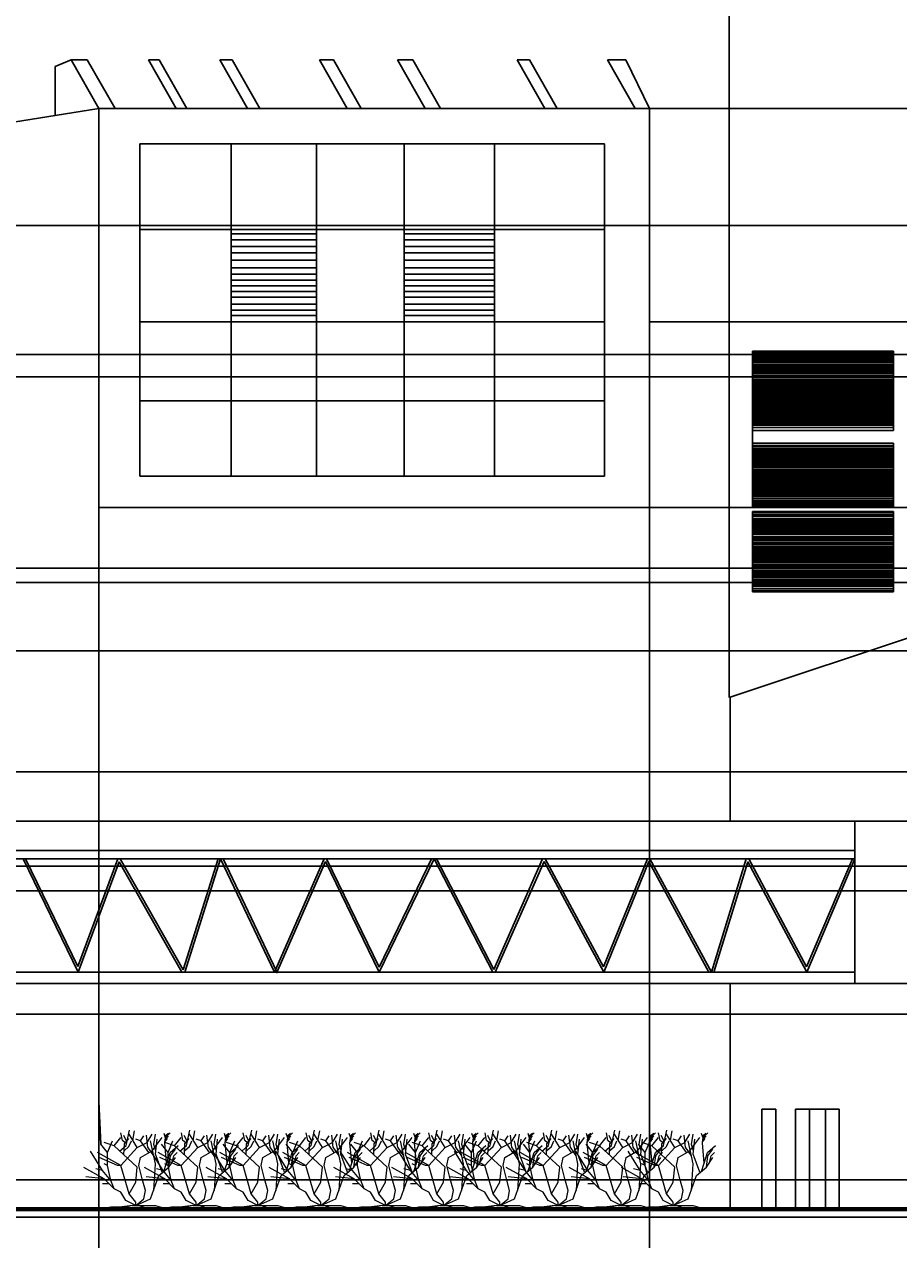
# Model space of a CAD drawing. Units: inches. Extents: x -32109 to 33221, y -19197 to 7608.
# Tile 20 of 25: x 12337 to 15375, y -2226 to 1998. Entities that reach past the tile are written whole.
import ezdxf

# ---------------------------------------------------------------- set-up
doc = ezdxf.new("R2010")
doc.units = ezdxf.units.IN
doc.header["$MEASUREMENT"] = 0
for name, color, linetype, lineweight in [('A-ANNO-DIMS', 2, 'Continuous', 18), ('A-ELEV', 7, 'Continuous', 25), ('L-PLNT', 3, 'Continuous', 13)]:
    doc.layers.add(name, color=color, linetype=linetype, lineweight=lineweight)
doc.styles.get("Standard").update_dxf_attribs({"font": 'arial.ttf'})
doc.dimstyles.get("Standard").update_dxf_attribs({"dimtxt": 0.18, "dimasz": 0.18, "dimexe": 0.18, "dimexo": 0.0625, "dimgap": 0.09, "dimtad": 0, "dimtih": 1, "dimtoh": 1, "dimdec": 4, "dimzin": 0, "dimdsep": 46, "dimtxsty": 'Standard', "dimcen": 0.09, "dimadec": 0, "dimazin": 0, "dimtfac": 1, "dimtdec": 4, "dimtofl": 0, "dimtmove": 0, "dimatfit": 3, "dimfxl": 1, "dimtolj": 1, "dimtzin": 0, "dimarcsym": 0})

# ---------------------------------------------------------------- blocks, each defined once
blk = doc.blocks.new('*U3')
for p, q in [((-12.471, 19.775), (-12.898, 22.044)), ((-11.28, 19.619), (-12.104, 21.184)), ((-11.433, 18.289), (-10.457, 22.749)), ((-8.16, 17.76), (-10.56, 21.6)), ((-9.48, 19.775), (-8.992, 22.592)), ((-5.086, 17.741), (-5.513, 21.34)), ((-5.28, 19.2), (-3.84, 21.6)), ((-3.377, 18.602), (-2.888, 21.575)), ((-0.508, 21.888), (-0.081, 20.558)), ((-0.203, 19.149), (0.102, 21.34)), ((0.041, 20.714), (1.384, 22.044)), ((0.102, 21.34), (0.835, 21.888)), ((-16.8, 16.32), (-18.72, 18.72)), ((-14.88, 18.24), (-17.76, 19.2)), ((-16.8, 16.32), (-15.36, 19.68)), ((-14.88, 18.24), (-12.96, 20.64)), ((-8.16, 12), (-14.88, 18.24)), ((-13.325, 16.724), (-11.433, 18.289)), ((-12.96, 12.48), (-8.16, 17.76)), ((-11.677, 19.071), (-12.471, 19.775)), ((-12.043, 15.628), (-11.921, 18.836)), ((-11.982, 16.802), (-10.579, 18.054)), ((-11.921, 18.836), (-10.64, 20.401)), ((-10.579, 18.054), (-9.846, 19.697)), ((-7.2, 19.68), (-8.64, 20.16)), ((-8.16, 17.76), (-5.28, 19.2)), ((-7.2, 19.68), (-6.24, 21.12)), ((-4.8, 16.32), (-7.2, 19.68)), ((-3.377, 15.315), (-5.086, 17.819)), ((-2.88, 12.96), (-4.32, 19.68)), ((-3.84, 16.8), (-0.96, 20.64)), ((-2.766, 16.802), (-3.377, 18.602)), ((-2.88, 15.84), (-2.4, 20.16)), ((0.346, 13.203), (-0.203, 19.149)), ((-0.142, 19.384), (0.59, 20.401)), ((-0.02, 20.01), (0.896, 21.105)), ((1.323, 16.254), (3.642, 18.289)), ((-18.24, 11.04), (-21.755, 16.655)), ((-12.96, 12.48), (-19.68, 16.32)), ((-13.92, 12.48), (-19.2, 14.88)), ((-16.8, 12.48), (-16.8, 16.32)), ((-7.68, 12.48), (-7.2, 14.88)), ((-7.2, 14.88), (-3.84, 16.8)), ((-0.96, 10.56), (-2.88, 15.84)), ((0.346, 13.203), (1.323, 16.254)), ((0.96, 12), (1.44, 15.36)), ((0.96, 12), (2.88, 14.88)), ((1.44, 15.36), (2.88, 17.28)), ((1.92, 13.44), (2.4, 15.36)), ((2.4, 15.36), (3.36, 16.32)), ((-17.76, 8.64), (-23.663, 11.961)), ((-18.24, 11.04), (-20.16, 11.52)), ((-15.84, 8.16), (-18.24, 11.04)), ((-16.8, 12.48), (-17.76, 12.96)), ((-15.84, 8.16), (-16.8, 12.48)), ((-12.96, 12.48), (-13.92, 12.48)), ((-10.56, 4.32), (-12.96, 12.48)), ((-8.64, 7.68), (-8.16, 12)), ((-6.72, 8.64), (-7.68, 12.48)), ((-3.36, 5.28), (-2.88, 12.96)), ((-1.92, 9.6), (0.96, 12)), ((-0.48, 10.8), (0.346, 13.203)), ((-17.76, 8.64), (-23.128, 9.222)), ((-16.32, 7.2), (-18.24, 7.2)), ((-14.88, 5.76), (-17.76, 8.64)), ((-14.88, 5.76), (-15.84, 8.16)), ((-10.56, 4.32), (-8.64, 7.68)), ((-5.76, 5.28), (-6.72, 8.64)), ((-4.32, 2.88), (-1.92, 9.6)), ((-12.96, 4.8), (-14.88, 5.76)), ((-11.52, 2.4), (-12.96, 4.8)), ((-8.64, 1.92), (-10.56, 4.32)), ((-6.24, 2.88), (-5.76, 5.28)), ((-15.84, 0.48), (-17.76, 0)), ((-13.44, 0.48), (-15.84, 0.48)), ((-9.6, 0.96), (-13.44, 0.48)), ((-9.6, 0.96), (-12.96, 0)), ((-8.64, 0.96), (-11.52, 2.4)), ((-9.6, 0.96), (-7.68, 0.96)), ((-8.64, 0.96), (-4.32, 2.88)), ((-8.64, 0.96), (-6.24, 2.88)), ((-8.64, 0.96), (-8.64, 1.92)), ((-8.64, 0.96), (-2.88, 0.96)), ((-7.68, 0.96), (-6.24, 0.48)), ((-6.24, 0.48), (-3.36, 0)), ((-2.88, 0.96), (0, 0))]:
    blk.add_line(p, q)
blk = doc.blocks.new('*D10')
at = {"layer": 'A-ANNO-DIMS', "color": 0, "lineweight": -2, "transparency": 16777216}
for p, q in [((-18512.6, -110.2), (-18512.6, 5772)), ((-18512.5, 5771.8), (-202.1, 5771.8)), ((18109.1, 5771.8), (-201.2, 5771.8)), ((18109.3, -101.5), (18109.3, 5772))]:
    blk.add_line(p, q, dxfattribs=at)
at = {"layer": 'A-ANNO-DIMS', "color": 0, "transparency": 16777216}
for points in [[(-18512.5, 5771.9), (-18512.5, 5771.8), (-18512.6, 5771.8)], [(18109.1, 5771.9), (18109.1, 5771.8), (18109.3, 5771.8)]]:
    blk.add_solid(points, dxfattribs=at)
at = {"layer": 'Defpoints', "color": 0, "transparency": 16777216}
for p in [(18109.3, 5771.8), (-18512.6, -110.2), (18109.3, -101.6)]:
    blk.add_point(p, dxfattribs=at)
at = {"layer": 'A-ANNO-DIMS', "color": 0, "transparency": 16777216, "insert": (-201.7, 5771.8), "char_height": 0.18, "attachment_point": 5}
blk.add_mtext('\\A1;36622', dxfattribs=at)
blk = doc.blocks.new('*D11')
at = {"layer": 'A-ANNO-DIMS', "color": 0, "lineweight": -2, "transparency": 16777216}
for p, q in [((14509.6, 1705.2), (25710.6, 1705.2)), ((25710.5, 1705), (25710.5, -209.6)), ((25710.5, -2124.6), (25710.5, -210)), ((-18512.6, -2124.8), (25710.6, -2124.8))]:
    blk.add_line(p, q, dxfattribs=at)
at = {"layer": 'A-ANNO-DIMS', "color": 0, "transparency": 16777216}
for points in [[(25710.4, 1705), (25710.5, 1705), (25710.5, 1705.2)], [(25710.4, -2124.6), (25710.5, -2124.6), (25710.5, -2124.8)]]:
    blk.add_solid(points, dxfattribs=at)
at = {"layer": 'Defpoints', "color": 0, "transparency": 16777216}
for p in [(14509.6, 1705.2), (-18512.6, -2124.8), (25710.5, -2124.8)]:
    blk.add_point(p, dxfattribs=at)
at = {"layer": 'A-ANNO-DIMS', "color": 0, "transparency": 16777216, "insert": (25710.5, -209.8), "char_height": 0.18, "attachment_point": 5}
blk.add_mtext('\\A1;3830', dxfattribs=at)
blk = doc.blocks.new('*D53')
at = {"layer": 'A-ANNO-DIMS', "color": 0, "lineweight": -2, "transparency": 16777216}
for p, q in [((-9508.3, -179.7), (25710.6, -179.7)), ((25710.5, -179.9), (25710.5, -389.7)), ((25710.5, -600), (25710.5, -390.1)), ((-9508.3, -600.2), (25710.6, -600.2))]:
    blk.add_line(p, q, dxfattribs=at)
at = {"layer": 'A-ANNO-DIMS', "color": 0, "transparency": 16777216}
for points in [[(25710.4, -179.9), (25710.5, -179.9), (25710.5, -179.7)], [(25710.4, -600), (25710.5, -600), (25710.5, -600.2)]]:
    blk.add_solid(points, dxfattribs=at)
at = {"layer": 'Defpoints', "color": 0, "transparency": 16777216}
for p in [(-9508.3, -179.7), (-9508.3, -600.2), (25710.5, -600.2)]:
    blk.add_point(p, dxfattribs=at)
at = {"layer": 'A-ANNO-DIMS', "color": 0, "transparency": 16777216, "insert": (25710.5, -389.9), "char_height": 0.18, "attachment_point": 5}
blk.add_mtext('\\A1;420.5', dxfattribs=at)
blk = doc.blocks.new('*D54')
at = {"layer": 'A-ANNO-DIMS', "color": 0, "lineweight": -2, "transparency": 16777216}
for p, q in [((-9508.3, -600.2), (25710.6, -600.2)), ((25710.5, -600.3), (25710.5, -806.8)), ((25710.5, -1013.7), (25710.5, -807.2)), ((-9508.3, -1013.9), (25710.6, -1013.9))]:
    blk.add_line(p, q, dxfattribs=at)
at = {"layer": 'A-ANNO-DIMS', "color": 0, "transparency": 16777216}
for points in [[(25710.4, -600.3), (25710.5, -600.3), (25710.5, -600.2)], [(25710.4, -1013.7), (25710.5, -1013.7), (25710.5, -1013.9)]]:
    blk.add_solid(points, dxfattribs=at)
at = {"layer": 'Defpoints', "color": 0, "transparency": 16777216}
for p in [(-9508.3, -600.2), (-9508.3, -1013.9), (25710.5, -1013.9)]:
    blk.add_point(p, dxfattribs=at)
at = {"layer": 'A-ANNO-DIMS', "color": 0, "transparency": 16777216, "insert": (25710.5, -807), "char_height": 0.18, "attachment_point": 5}
blk.add_mtext('\\A1;413.7', dxfattribs=at)
blk = doc.blocks.new('*D55')
at = {"layer": 'A-ANNO-DIMS', "color": 0, "lineweight": -2, "transparency": 16777216}
for p, q in [((-9508.3, -1013.9), (25710.6, -1013.9)), ((25710.5, -1014.1), (25710.5, -1227.7)), ((25710.5, -1441.6), (25710.5, -1228)), ((-9508.3, -1441.8), (25710.6, -1441.8))]:
    blk.add_line(p, q, dxfattribs=at)
at = {"layer": 'A-ANNO-DIMS', "color": 0, "transparency": 16777216}
for points in [[(25710.4, -1014.1), (25710.5, -1014.1), (25710.5, -1013.9)], [(25710.4, -1441.6), (25710.5, -1441.6), (25710.5, -1441.8)]]:
    blk.add_solid(points, dxfattribs=at)
at = {"layer": 'Defpoints', "color": 0, "transparency": 16777216}
for p in [(-9508.3, -1013.9), (-9508.3, -1441.8), (25710.5, -1441.8)]:
    blk.add_point(p, dxfattribs=at)
at = {"layer": 'A-ANNO-DIMS', "color": 0, "transparency": 16777216, "insert": (25710.5, -1227.9), "char_height": 0.18, "attachment_point": 5}
blk.add_mtext('\\A1;427.9', dxfattribs=at)
blk = doc.blocks.new('*D56')
at = {"layer": 'A-ANNO-DIMS', "color": 0, "lineweight": -2, "transparency": 16777216}
for p, q in [((-9508.3, -1441.8), (25710.6, -1441.8)), ((25710.5, -1442), (25710.5, -1730.1)), ((25710.5, -2018.6), (25710.5, -1730.5)), ((-9508.3, -2018.8), (25710.6, -2018.8))]:
    blk.add_line(p, q, dxfattribs=at)
at = {"layer": 'A-ANNO-DIMS', "color": 0, "transparency": 16777216}
for points in [[(25710.4, -1442), (25710.5, -1442), (25710.5, -1441.8)], [(25710.4, -2018.6), (25710.5, -2018.6), (25710.5, -2018.8)]]:
    blk.add_solid(points, dxfattribs=at)
at = {"layer": 'Defpoints', "color": 0, "transparency": 16777216}
for p in [(-9508.3, -1441.8), (-9508.3, -2018.8), (25710.5, -2018.8)]:
    blk.add_point(p, dxfattribs=at)
at = {"layer": 'A-ANNO-DIMS', "color": 0, "transparency": 16777216, "insert": (25710.5, -1730.3), "char_height": 0.18, "attachment_point": 5}
blk.add_mtext('\\A1;576.9', dxfattribs=at)
blk = doc.blocks.new('*D62')
at = {"layer": 'A-ANNO-DIMS', "color": 0, "lineweight": -2, "transparency": 16777216}
for p, q in [((12596.6, 1705.1), (12596.6, -5429.7)), ((11383.7, -2116.2), (11383.7, -5429.7)), ((11383.9, -5429.6), (11989.8, -5429.6)), ((12596.5, -5429.6), (11990.5, -5429.6))]:
    blk.add_line(p, q, dxfattribs=at)
at = {"layer": 'A-ANNO-DIMS', "color": 0, "transparency": 16777216}
for points in [[(11383.9, -5429.5), (11383.9, -5429.6), (11383.7, -5429.6)], [(12596.5, -5429.5), (12596.5, -5429.6), (12596.6, -5429.6)]]:
    blk.add_solid(points, dxfattribs=at)
at = {"layer": 'Defpoints', "color": 0, "transparency": 16777216}
for p in [(12596.6, 1705.2), (11383.7, -2116.1), (12596.6, -5429.6)]:
    blk.add_point(p, dxfattribs=at)
at = {"layer": 'A-ANNO-DIMS', "color": 0, "transparency": 16777216, "insert": (11990.2, -5429.6), "char_height": 0.18, "attachment_point": 5}
blk.add_mtext('\\A1;1213', dxfattribs=at)
blk = doc.blocks.new('*D63')
at = {"layer": 'A-ANNO-DIMS', "color": 0, "lineweight": -2, "transparency": 16777216}
for p, q in [((12596.6, 1705.1), (12596.6, -5429.7)), ((14509.6, 1705.1), (14509.6, -5429.7)), ((12596.8, -5429.6), (13552.7, -5429.6)), ((14509.4, -5429.6), (13553.4, -5429.6))]:
    blk.add_line(p, q, dxfattribs=at)
at = {"layer": 'A-ANNO-DIMS', "color": 0, "transparency": 16777216}
for points in [[(12596.8, -5429.5), (12596.8, -5429.6), (12596.6, -5429.6)], [(14509.4, -5429.5), (14509.4, -5429.6), (14509.6, -5429.6)]]:
    blk.add_solid(points, dxfattribs=at)
at = {"layer": 'Defpoints', "color": 0, "transparency": 16777216}
for p in [(12596.6, 1705.2), (14509.6, 1705.2), (14509.6, -5429.6)]:
    blk.add_point(p, dxfattribs=at)
at = {"layer": 'A-ANNO-DIMS', "color": 0, "transparency": 16777216, "insert": (13553.1, -5429.6), "char_height": 0.18, "attachment_point": 5}
blk.add_mtext('\\A1;1913', dxfattribs=at)
blk = doc.blocks.new('*D64')
at = {"layer": 'A-ANNO-DIMS', "color": 0, "lineweight": -2, "transparency": 16777216}
for p, q in [((14509.6, 1705.1), (14509.6, -5429.7)), ((15505.7, -101.7), (15505.7, -5429.7)), ((14509.7, -5429.6), (15007.3, -5429.6)), ((15505.6, -5429.6), (15008, -5429.6))]:
    blk.add_line(p, q, dxfattribs=at)
at = {"layer": 'A-ANNO-DIMS', "color": 0, "transparency": 16777216}
for points in [[(14509.7, -5429.5), (14509.7, -5429.6), (14509.6, -5429.6)], [(15505.6, -5429.5), (15505.6, -5429.6), (15505.7, -5429.6)]]:
    blk.add_solid(points, dxfattribs=at)
at = {"layer": 'Defpoints', "color": 0, "transparency": 16777216}
for p in [(14509.6, 1705.2), (15505.7, -101.6), (15505.7, -5429.6)]:
    blk.add_point(p, dxfattribs=at)
at = {"layer": 'A-ANNO-DIMS', "color": 0, "transparency": 16777216, "insert": (15007.6, -5429.6), "char_height": 0.18, "attachment_point": 5}
blk.add_mtext('\\A1;996.2', dxfattribs=at)
blk = doc.blocks.new('*D66')
at = {"layer": 'A-ANNO-DIMS', "color": 0, "lineweight": -2, "transparency": 16777216}
for p, q in [((14786.4, 963.8), (14786.4, 5772)), ((14786.6, 5771.8), (15747.7, 5771.8)), ((16709.6, 5771.8), (15748.6, 5771.8)), ((16709.8, 963.8), (16709.8, 5772))]:
    blk.add_line(p, q, dxfattribs=at)
at = {"layer": 'A-ANNO-DIMS', "color": 0, "transparency": 16777216}
for points in [[(14786.6, 5771.9), (14786.6, 5771.8), (14786.4, 5771.8)], [(16709.6, 5771.9), (16709.6, 5771.8), (16709.8, 5771.8)]]:
    blk.add_solid(points, dxfattribs=at)
at = {"layer": 'Defpoints', "color": 0, "transparency": 16777216}
for p in [(16709.8, 5771.8), (14786.4, 963.7), (16709.8, 963.7)]:
    blk.add_point(p, dxfattribs=at)
at = {"layer": 'A-ANNO-DIMS', "color": 0, "transparency": 16777216, "insert": (15748.1, 5771.8), "char_height": 0.18, "attachment_point": 5}
blk.add_mtext('\\A1;1923.4', dxfattribs=at)
blk = doc.blocks.new('*D67')
at = {"layer": 'A-ANNO-DIMS', "color": 0, "lineweight": -2, "transparency": 16777216}
for p, q in [((1645.9, 851.2), (25710.6, 851.2)), ((25710.5, 851), (25710.5, -632.3)), ((25710.5, -2116), (25710.5, -632.7)), ((1588.2, -2116.1), (25710.6, -2116.1))]:
    blk.add_line(p, q, dxfattribs=at)
at = {"layer": 'A-ANNO-DIMS', "color": 0, "transparency": 16777216}
for points in [[(25710.4, 851), (25710.5, 851), (25710.5, 851.2)], [(25710.4, -2116), (25710.5, -2116), (25710.5, -2116.1)]]:
    blk.add_solid(points, dxfattribs=at)
at = {"layer": 'Defpoints', "color": 0, "transparency": 16777216}
for p in [(1645.8, 851.2), (1588.2, -2116.1), (25710.5, -2116.1)]:
    blk.add_point(p, dxfattribs=at)
at = {"layer": 'A-ANNO-DIMS', "color": 0, "transparency": 16777216, "insert": (25710.5, -632.5), "char_height": 0.18, "attachment_point": 5}
blk.add_mtext('\\A1;2967.4', dxfattribs=at)
blk = doc.blocks.new('*D68')
at = {"layer": 'A-ANNO-DIMS', "color": 0, "lineweight": -2, "transparency": 16777216}
for p, q in [((4084.1, -927.5), (25710.6, -927.5)), ((25710.5, -927.7), (25710.5, -1521.6)), ((25710.5, -2116), (25710.5, -1522)), ((4084.1, -2116.1), (25710.6, -2116.1))]:
    blk.add_line(p, q, dxfattribs=at)
at = {"layer": 'A-ANNO-DIMS', "color": 0, "transparency": 16777216}
for points in [[(25710.4, -927.7), (25710.5, -927.7), (25710.5, -927.5)], [(25710.4, -2116), (25710.5, -2116), (25710.5, -2116.1)]]:
    blk.add_solid(points, dxfattribs=at)
at = {"layer": 'Defpoints', "color": 0, "transparency": 16777216}
for p in [(4084, -927.5), (4084, -2116.1), (25710.5, -2116.1)]:
    blk.add_point(p, dxfattribs=at)
at = {"layer": 'A-ANNO-DIMS', "color": 0, "transparency": 16777216, "insert": (25710.5, -1521.8), "char_height": 0.18, "attachment_point": 5}
blk.add_mtext('\\A1;1188.7', dxfattribs=at)
blk = doc.blocks.new('*D69')
at = {"layer": 'A-ANNO-DIMS', "color": 0, "lineweight": -2, "transparency": 16777216}
for p, q in [((5273.8, 1298.7), (25710.6, 1298.7)), ((25710.5, 1298.5), (25710.5, -411.9)), ((25710.5, -2122.6), (25710.5, -412.2)), ((5279.3, -2122.7), (25710.6, -2122.7))]:
    blk.add_line(p, q, dxfattribs=at)
at = {"layer": 'A-ANNO-DIMS', "color": 0, "transparency": 16777216}
for points in [[(25710.4, 1298.5), (25710.5, 1298.5), (25710.5, 1298.7)], [(25710.4, -2122.6), (25710.5, -2122.6), (25710.5, -2122.7)]]:
    blk.add_solid(points, dxfattribs=at)
at = {"layer": 'Defpoints', "color": 0, "transparency": 16777216}
for p in [(5273.7, 1298.7), (5279.3, -2122.7), (25710.5, -2122.7)]:
    blk.add_point(p, dxfattribs=at)
at = {"layer": 'A-ANNO-DIMS', "color": 0, "transparency": 16777216, "insert": (25710.5, -412), "char_height": 0.18, "attachment_point": 5}
blk.add_mtext('\\A1;3421.4', dxfattribs=at)
blk = doc.blocks.new('*D70')
at = {"layer": 'A-ANNO-DIMS', "color": 0, "lineweight": -2, "transparency": 16777216}
for p, q in [((8883.3, 57.8), (25710.6, 57.8)), ((25710.5, 57.6), (25710.5, -1045.1)), ((25710.5, -2148.2), (25710.5, -1045.5)), ((8832.4, -2148.4), (25710.6, -2148.4))]:
    blk.add_line(p, q, dxfattribs=at)
at = {"layer": 'A-ANNO-DIMS', "color": 0, "transparency": 16777216}
for points in [[(25710.4, 57.6), (25710.5, 57.6), (25710.5, 57.8)], [(25710.4, -2148.2), (25710.5, -2148.2), (25710.5, -2148.4)]]:
    blk.add_solid(points, dxfattribs=at)
at = {"layer": 'Defpoints', "color": 0, "transparency": 16777216}
for p in [(8883.2, 57.8), (8832.3, -2148.4), (25710.5, -2148.4)]:
    blk.add_point(p, dxfattribs=at)
at = {"layer": 'A-ANNO-DIMS', "color": 0, "transparency": 16777216, "insert": (25710.5, -1045.3), "char_height": 0.18, "attachment_point": 5}
blk.add_mtext('\\A1;2206', dxfattribs=at)
blk = doc.blocks.new('*D71')
at = {"layer": 'A-ANNO-DIMS', "color": 0, "lineweight": -2, "transparency": 16777216}
for p, q in [((11823.3, 772.8), (25710.6, 772.8)), ((25710.5, 772.6), (25710.5, 440.5)), ((25710.5, 107.9), (25710.5, 440.1)), ((11823.3, 107.7), (25710.6, 107.7))]:
    blk.add_line(p, q, dxfattribs=at)
at = {"layer": 'A-ANNO-DIMS', "color": 0, "transparency": 16777216}
for points in [[(25710.4, 772.6), (25710.5, 772.6), (25710.5, 772.8)], [(25710.4, 107.9), (25710.5, 107.9), (25710.5, 107.7)]]:
    blk.add_solid(points, dxfattribs=at)
at = {"layer": 'Defpoints', "color": 0, "transparency": 16777216}
for p in [(11823.2, 772.8), (11823.2, 107.7), (25710.5, 107.7)]:
    blk.add_point(p, dxfattribs=at)
at = {"layer": 'A-ANNO-DIMS', "color": 0, "transparency": 16777216, "insert": (25710.5, 440.3), "char_height": 0.18, "attachment_point": 5}
blk.add_mtext('\\A1;665.1', dxfattribs=at)
blk = doc.blocks.new('*D72')
at = {"layer": 'A-ANNO-DIMS', "color": 0, "lineweight": -2, "transparency": 16777216}
for p, q in [((11823.3, 107.7), (25710.6, 107.7)), ((25710.5, 107.6), (25710.5, -1004)), ((25710.5, -2116), (25710.5, -1004.4)), ((11383.7, -2116.1), (25710.6, -2116.1))]:
    blk.add_line(p, q, dxfattribs=at)
at = {"layer": 'A-ANNO-DIMS', "color": 0, "transparency": 16777216}
for points in [[(25710.4, 107.6), (25710.5, 107.6), (25710.5, 107.7)], [(25710.4, -2116), (25710.5, -2116), (25710.5, -2116.1)]]:
    blk.add_solid(points, dxfattribs=at)
at = {"layer": 'Defpoints', "color": 0, "transparency": 16777216}
for p in [(11823.2, 107.7), (11383.7, -2116.1), (25710.5, -2116.1)]:
    blk.add_point(p, dxfattribs=at)
at = {"layer": 'A-ANNO-DIMS', "color": 0, "transparency": 16777216, "insert": (25710.5, -1004.2), "char_height": 0.18, "attachment_point": 5}
blk.add_mtext('\\A1;2224', dxfattribs=at)
blk = doc.blocks.new('*D74')
at = {"layer": 'A-ANNO-DIMS', "color": 0, "lineweight": -2, "transparency": 16777216}
for p, q in [((15223.2, -771.9), (25710.6, -771.9)), ((25710.5, -772.1), (25710.5, -1053.6)), ((25710.5, -1335.5), (25710.5, -1054)), ((15223.2, -1335.7), (25710.6, -1335.7))]:
    blk.add_line(p, q, dxfattribs=at)
at = {"layer": 'A-ANNO-DIMS', "color": 0, "transparency": 16777216}
for points in [[(25710.4, -772.1), (25710.5, -772.1), (25710.5, -771.9)], [(25710.4, -1335.5), (25710.5, -1335.5), (25710.5, -1335.7)]]:
    blk.add_solid(points, dxfattribs=at)
at = {"layer": 'Defpoints', "color": 0, "transparency": 16777216}
for p in [(15223.2, -771.9), (15223.2, -1335.7), (25710.5, -1335.7)]:
    blk.add_point(p, dxfattribs=at)
at = {"layer": 'A-ANNO-DIMS', "color": 0, "transparency": 16777216, "insert": (25710.5, -1053.8), "char_height": 0.18, "attachment_point": 5}
blk.add_mtext('\\A1;563.8', dxfattribs=at)
blk = doc.blocks.new('*D75')
at = {"layer": 'A-ANNO-DIMS', "color": 0, "lineweight": -2, "transparency": 16777216}
for p, q in [((14509.6, 1705.2), (25710.6, 1705.2)), ((25710.5, 1705), (25710.5, 1012.4)), ((25710.5, 319.4), (25710.5, 1012)), ((14509.6, 319.2), (25710.6, 319.2))]:
    blk.add_line(p, q, dxfattribs=at)
at = {"layer": 'A-ANNO-DIMS', "color": 0, "transparency": 16777216}
for points in [[(25710.4, 1705), (25710.5, 1705), (25710.5, 1705.2)], [(25710.4, 319.4), (25710.5, 319.4), (25710.5, 319.2)]]:
    blk.add_solid(points, dxfattribs=at)
at = {"layer": 'Defpoints', "color": 0, "transparency": 16777216}
for p in [(14509.6, 1705.2), (14509.6, 319.2), (25710.5, 319.2)]:
    blk.add_point(p, dxfattribs=at)
at = {"layer": 'A-ANNO-DIMS', "color": 0, "transparency": 16777216, "insert": (25710.5, 1012.2), "char_height": 0.18, "attachment_point": 5}
blk.add_mtext('\\A1;1386', dxfattribs=at)

msp = doc.modelspace()

# ---------------------------------------------------------------- linework, layer by layer
at = {"layer": 'A-ELEV'}
for p, q in [((12500.298, 1874.823), (12444.346, 1851.216)), ((12596.642, 1705.162), (12500.298, 1874.823)), ((12500.298, 1874.823), (12556.111, 1874.823)), ((12652.455, 1705.162), (12556.111, 1874.823)), ((12864.599, 1705.162), (12768.254, 1874.823)), ((12768.254, 1874.823), (12806.089, 1874.823)), ((12902.433, 1705.162), (12806.089, 1874.823)), ((13112.431, 1705.162), (13016.086, 1874.823)), ((13016.086, 1874.823), (13059.033, 1874.823)), ((13155.378, 1705.162), (13059.033, 1874.823)), ((13459.14, 1705.162), (13362.795, 1874.823)), ((13362.795, 1874.823), (13411.439, 1874.823)), ((13507.784, 1705.162), (13411.439, 1874.823)), ((13729.789, 1705.162), (13633.444, 1874.823)), ((13633.444, 1874.823), (13687.127, 1874.823)), ((13783.472, 1705.162), (13687.127, 1874.823)), ((14145.564, 1705.162), (14049.219, 1874.823)), ((14049.219, 1874.823), (14092.459, 1874.823)), ((14188.803, 1705.162), (14092.459, 1874.823)), ((14459.881, 1705.162), (14363.537, 1874.823)), ((14363.537, 1874.823), (14426.744, 1874.823)), ((14426.744, 1874.823), (14509.55, 1705.162)), ((12444.346, 1851.216), (12444.346, 1681.095)), ((11819.608, 1582.37), (12596.642, 1705.162)), ((12596.642, 1705.162), (12596.642, 319.218)), ((14509.55, 1705.162), (12596.642, 1705.162)), ((14509.55, 319.218), (14509.55, 1705.162)), ((12738.402, 427.912), (12738.402, 1583.272)), ((12738.402, 1583.272), (14352.499, 1583.272)), ((13056.292, 427.912), (13056.292, 1583.272)), ((13056.292, 1583.272), (13352.23, 1583.272)), ((13352.23, 427.912), (13352.23, 1583.272)), ((13657.136, 427.912), (13657.136, 1583.272)), ((13971.009, 427.912), (13971.009, 1583.272)), ((14352.499, 1583.272), (14352.499, 427.912)), ((12738.402, 1284.952), (14352.499, 1284.952)), ((13056.292, 1269.983), (13352.23, 1269.983)), ((13657.136, 1269.983), (13971.009, 1269.983)), ((13056.292, 1248.675), (13352.23, 1248.675)), ((13056.292, 1226.623), (13352.23, 1226.623)), ((13657.136, 1248.675), (13971.009, 1248.675)), ((13657.136, 1226.623), (13971.009, 1226.623)), ((13056.292, 1204.401), (13352.23, 1204.401)), ((13657.136, 1204.401), (13971.009, 1204.401)), ((13056.292, 1178.927), (13352.23, 1178.927)), ((13056.292, 1151.828), (13352.23, 1151.828)), ((13657.136, 1178.927), (13971.009, 1178.927)), ((13657.136, 1151.828), (13971.009, 1151.828)), ((13056.292, 1129.963), (13352.23, 1129.963)), ((13056.292, 1109.367), (13352.23, 1109.367)), ((13657.136, 1129.963), (13971.009, 1129.963)), ((13657.136, 1109.367), (13971.009, 1109.367)), ((13056.292, 1089.313), (13352.23, 1089.313)), ((13056.292, 1069.259), (13352.23, 1069.259)), ((13657.136, 1089.313), (13971.009, 1089.313)), ((13657.136, 1069.259), (13971.009, 1069.259)), ((13056.292, 1050.29), (13352.23, 1050.29)), ((13056.292, 1025.335), (13352.23, 1025.335)), ((13657.136, 1050.29), (13971.009, 1050.29)), ((13657.136, 1025.335), (13971.009, 1025.335)), ((13056.292, 1004.259), (13352.23, 1004.259)), ((13056.292, 986.243), (13352.23, 986.243)), ((13657.136, 1004.259), (13971.009, 1004.259)), ((13657.136, 986.243), (13971.009, 986.243)), ((12738.402, 964.741), (14352.499, 964.741)), ((14511.797, 963.73), (14786.396, 963.73)), ((14786.396, 963.73), (14786.396, -101.6)), ((14786.396, 963.73), (16709.825, 963.73)), ((14867.272, 862.63), (15356.79, 862.63)), ((14867.272, 322.086), (14867.272, 862.63)), ((14867.272, 858.462), (15356.79, 858.462)), ((14867.272, 855.612), (15356.79, 855.612)), ((14867.272, 849.733), (15356.79, 849.733)), ((14867.272, 845.261), (15356.79, 845.261)), ((15356.79, 586.032), (15356.79, 862.63)), ((14867.272, 841.894), (15356.79, 841.894)), ((14867.272, 837.975), (15356.79, 837.975)), ((14867.272, 834.701), (15356.79, 834.701)), ((14867.272, 832.095), (15356.79, 832.095)), ((14867.272, 827.66), (15356.79, 827.66)), ((14867.272, 826.216), (15356.79, 826.216)), ((14867.272, 822.38), (15356.79, 822.38)), ((14867.272, 822.297), (15356.79, 822.297)), ((14867.272, 816.418), (15356.79, 816.418)), ((14867.272, 810.538), (15356.79, 810.538)), ((14867.272, 806.619), (15356.79, 806.619)), ((14867.272, 800.74), (15356.79, 800.74)), ((14867.272, 796.82), (15356.79, 796.82)), ((14867.272, 794.218), (15356.79, 794.218)), ((14867.272, 792.901), (15356.79, 792.901)), ((14867.272, 787.022), (15356.79, 787.022)), ((14867.272, 785.418), (15356.79, 785.418)), ((14867.272, 779.183), (15356.79, 779.183)), ((14867.272, 775.737), (15356.79, 775.737)), ((14867.272, 775.737), (15356.79, 775.737)), ((14867.272, 771.344), (15356.79, 771.344)), ((14867.272, 765.176), (15356.79, 765.176)), ((14867.272, 762.684), (15356.79, 762.684)), ((14867.272, 758.136), (15356.79, 758.136)), ((14867.272, 755.666), (15356.79, 755.666)), ((14867.272, 752.856), (15356.79, 752.856)), ((14867.272, 749.787), (15356.79, 749.787)), ((14867.272, 746.695), (15356.79, 746.695)), ((14867.272, 741.948), (15356.79, 741.948)), ((14867.272, 738.775), (15356.79, 738.775)), ((14867.272, 738.029), (15356.79, 738.029)), ((14867.272, 732.614), (15356.79, 732.614)), ((14867.272, 732.15), (15356.79, 732.15)), ((14867.272, 726.27), (15356.79, 726.27)), ((14867.272, 722.934), (15356.79, 722.934)), ((14867.272, 722.351), (15356.79, 722.351)), ((12738.402, 689.471), (14352.499, 689.471)), ((14867.272, 716.774), (15356.79, 716.774)), ((14867.272, 716.472), (15356.79, 716.472)), ((14867.272, 710.593), (15356.79, 710.593)), ((14867.272, 709.733), (15356.79, 709.733)), ((14867.272, 706.673), (15356.79, 706.673)), ((14867.272, 700.794), (15356.79, 700.794)), ((14867.272, 697.412), (15356.79, 697.412)), ((14867.272, 696.875), (15356.79, 696.875)), ((14867.272, 694.772), (15356.79, 694.772)), ((14867.272, 692.955), (15356.79, 692.955)), ((14867.272, 687.076), (15356.79, 687.076)), ((14867.272, 685.972), (15356.79, 685.972)), ((14867.272, 684.212), (15356.79, 684.212)), ((14867.272, 680.376), (15356.79, 680.376)), ((14867.272, 679.237), (15356.79, 679.237)), ((14867.272, 673.358), (15356.79, 673.358)), ((14867.272, 671.398), (15356.79, 671.398)), ((14867.272, 667.479), (15356.79, 667.479)), ((14867.272, 663.09), (15356.79, 663.09)), ((14867.272, 660.45), (15356.79, 660.45)), ((14867.272, 659.64), (15356.79, 659.64)), ((14867.272, 655.72), (15356.79, 655.72)), ((14867.272, 649.89), (15356.79, 649.89)), ((14867.272, 649.841), (15356.79, 649.841)), ((14867.272, 643.962), (15356.79, 643.962)), ((14867.272, 640.043), (15356.79, 640.043)), ((14867.272, 634.163), (15356.79, 634.163)), ((14867.272, 628.284), (15356.79, 628.284)), ((14867.272, 624.365), (15356.79, 624.365)), ((14867.272, 618.486), (15356.79, 618.486)), ((14867.272, 614.566), (15356.79, 614.566)), ((14867.272, 610.647), (15356.79, 610.647)), ((14867.272, 604.768), (15356.79, 604.768)), ((14867.272, 596.929), (15356.79, 596.929)), ((14867.272, 586.032), (15356.79, 586.032)), ((14867.272, 542.056), (15356.79, 542.056)), ((14867.272, 534.218), (15356.79, 534.218)), ((14867.272, 530.298), (15356.79, 530.298)), ((14867.272, 524.419), (15356.79, 524.419)), ((14867.272, 518.54), (15356.79, 518.54)), ((14867.272, 514.62), (15356.79, 514.62)), ((14867.272, 508.741), (15356.79, 508.741)), ((15356.79, 322.086), (15356.79, 542.056)), ((14867.272, 502.862), (15356.79, 502.862)), ((14867.272, 498.943), (15356.79, 498.943)), ((14867.272, 493.063), (15356.79, 493.063)), ((14867.272, 489.144), (15356.79, 489.144)), ((14867.272, 485.224), (15356.79, 485.224)), ((14867.272, 479.871), (15356.79, 479.871)), ((14867.272, 479.345), (15356.79, 479.345)), ((14867.272, 474.201), (15356.79, 474.201)), ((14867.272, 474.201), (15356.79, 474.201)), ((14867.272, 471.506), (15356.79, 471.506)), ((14867.272, 467.113), (15356.79, 467.113)), ((14867.272, 465.695), (15356.79, 465.695)), ((12738.402, 427.912), (14352.499, 427.912)), ((14867.272, 463.668), (15356.79, 463.668)), ((14867.272, 460.025), (15356.79, 460.025)), ((14867.272, 456.968), (15356.79, 456.968)), ((14867.272, 449.949), (15356.79, 449.949)), ((14867.272, 447.267), (15356.79, 447.267)), ((14867.272, 447.267), (15356.79, 447.267)), ((14867.272, 444.07), (15356.79, 444.07)), ((14867.272, 438.762), (15356.79, 438.762)), ((14867.272, 438.762), (15356.79, 438.762)), ((14867.272, 436.231), (15356.79, 436.231)), ((14867.272, 434.509), (15356.79, 434.509)), ((14867.272, 432.312), (15356.79, 432.312)), ((14867.272, 431.674), (15356.79, 431.674)), ((14867.272, 426.433), (15356.79, 426.433)), ((14867.272, 423.169), (15356.79, 423.169)), ((14867.272, 420.554), (15356.79, 420.554)), ((14867.272, 416.634), (15356.79, 416.634)), ((14867.272, 413.246), (15356.79, 413.246)), ((14867.272, 410.755), (15356.79, 410.755)), ((14867.272, 407.576), (15356.79, 407.576)), ((14867.272, 404.876), (15356.79, 404.876)), ((14867.272, 400.956), (15356.79, 400.956)), ((14867.272, 395.077), (15356.79, 395.077)), ((14867.272, 391.158), (15356.79, 391.158)), ((14867.272, 387.238), (15356.79, 387.238)), ((14867.272, 381.359), (15356.79, 381.359)), ((14867.272, 378.34), (15356.79, 378.34)), ((14867.272, 373.52), (15356.79, 373.52)), ((14867.272, 369.974), (15356.79, 369.974)), ((14867.272, 365.681), (15356.79, 365.681)), ((14867.272, 365.681), (15325.097, 365.681)), ((14867.272, 365.681), (15329.355, 365.681)), ((14867.272, 365.681), (15323.678, 365.681)), ((14867.272, 365.681), (15320.839, 365.681)), ((14867.272, 365.681), (15325.097, 365.681)), ((14867.272, 360.793), (15356.79, 360.793)), ((14867.272, 356.219), (15356.79, 356.219)), ((14867.272, 348.564), (15356.79, 348.564)), ((14867.272, 341.652), (15356.79, 341.652)), ((12596.642, 319.218), (12738.402, 319.218)), ((12596.642, 319.218), (14509.55, 319.218)), ((12596.642, -101.6), (12596.642, 319.218)), ((14352.499, 319.218), (14509.55, 319.218)), ((14867.272, 337.398), (15356.79, 337.398)), ((14867.272, 332.612), (15356.79, 332.612)), ((14867.272, 326.763), (15356.79, 326.763)), ((14867.272, 322.086), (15356.79, 322.086)), ((14867.272, 25.622), (14867.272, 305.269)), ((14867.272, 305.269), (15356.79, 305.269)), ((14867.272, 301.434), (15356.79, 301.434)), ((15356.79, 25.622), (15356.79, 305.269)), ((14867.272, 294.416), (15356.79, 294.416)), ((14867.272, 288.537), (15356.79, 288.537)), ((14867.272, 280.698), (15356.79, 280.698)), ((14867.272, 276.778), (15356.79, 276.778)), ((14867.272, 270.899), (15356.79, 270.899)), ((14867.272, 265.02), (15356.79, 265.02)), ((14867.272, 261.101), (15356.79, 261.101)), ((14867.272, 255.221), (15356.79, 255.221)), ((14867.272, 249.342), (15356.79, 249.342)), ((14867.272, 245.423), (15356.79, 245.423)), ((14867.272, 239.544), (15356.79, 239.544)), ((14867.272, 235.624), (15356.79, 235.624)), ((14867.272, 234.635), (15356.79, 234.635)), ((14867.272, 231.705), (15356.79, 231.705)), ((14867.272, 225.826), (15356.79, 225.826)), ((14867.272, 217.987), (15356.79, 217.987)), ((14867.272, 211.954), (15356.79, 211.954)), ((14867.272, 210.536), (15356.79, 210.536)), ((14867.272, 210.148), (15356.79, 210.148)), ((14867.272, 206.284), (15356.79, 206.284)), ((14867.272, 206.284), (15356.79, 206.284)), ((14867.272, 203.448), (15356.79, 203.448)), ((14867.272, 196.43), (15356.79, 196.43)), ((14867.272, 196.361), (15356.79, 196.361)), ((14867.272, 190.551), (15356.79, 190.551)), ((14867.272, 182.712), (15356.79, 182.712)), ((14867.272, 178.792), (15356.79, 178.792)), ((14867.272, 172.913), (15356.79, 172.913)), ((14867.272, 167.034), (15356.79, 167.034)), ((14867.272, 163.757), (15356.79, 163.757)), ((14867.272, 163.114), (15356.79, 163.114)), ((14867.272, 157.235), (15356.79, 157.235)), ((14867.272, 156.67), (15356.79, 156.67)), ((14867.272, 151.356), (15356.79, 151.356)), ((14867.272, 147.437), (15356.79, 147.437)), ((14867.272, 141.558), (15356.79, 141.558)), ((14867.272, 137.638), (15356.79, 137.638)), ((14867.272, 135.406), (15356.79, 135.406)), ((14867.272, 133.719), (15356.79, 133.719)), ((14867.272, 128.319), (15356.79, 128.319)), ((14867.272, 127.839), (15356.79, 127.839)), ((14867.272, 121.14), (15356.79, 121.14)), ((14867.272, 120.001), (15356.79, 120.001)), ((14867.272, 119.813), (15356.79, 119.813)), ((14867.272, 114.121), (15356.79, 114.121)), ((14867.272, 112.162), (15356.79, 112.162)), ((14867.272, 108.242), (15356.79, 108.242)), ((14867.272, 100.403), (15356.79, 100.403)), ((14867.272, 96.484), (15356.79, 96.484)), ((14867.272, 90.605), (15356.79, 90.605)), ((14867.272, 84.726), (15356.79, 84.726)), ((14867.272, 80.806), (15356.79, 80.806)), ((14867.272, 74.927), (15356.79, 74.927)), ((14867.272, 69.048), (15356.79, 69.048)), ((14867.272, 65.128), (15356.79, 65.128)), ((14867.272, 59.249), (15356.79, 59.249)), ((14867.272, 55.33), (15356.79, 55.33)), ((14867.272, 51.41), (15356.79, 51.41)), ((14867.272, 45.531), (15356.79, 45.531)), ((14867.272, 37.692), (15356.79, 37.692)), ((14867.272, 29.853), (15356.79, 29.853)), ((15356.79, 25.622), (14867.272, 25.622)), ((12596.642, -101.6), (12596.642, -771.886)), ((15505.744, -101.6), (14786.396, -341.579)), ((14786.396, -101.6), (14786.396, -341.579)), ((14789.269, -340.62), (14789.269, -771.886)), ((11384.05, -771.886), (15223.17, -771.886)), ((15223.17, -771.886), (15223.17, -873.541)), ((15223.17, -873.541), (11398.466, -873.541)), ((15223.17, -902.193), (15223.17, -873.541)), ((11398.466, -902.193), (15223.17, -902.193)), ((12333.137, -902.926), (12524.495, -1296.425)), ((12341.549, -902.193), (12523.511, -1276.372)), ((12523.511, -1276.372), (12662.031, -902.193)), ((12524.495, -1296.425), (12666.559, -912.674)), ((12666.559, -912.674), (12884.314, -1296.295)), ((12670.138, -903.007), (12888.83, -1288.278)), ((12888.83, -1288.278), (13011.102, -902.193)), ((12894.562, -1296.295), (13019.206, -902.721)), ((13019.206, -902.721), (13206.357, -1296.5)), ((13027.686, -902.193), (13213.478, -1293.115)), ((13206.357, -1296.5), (13378.7, -902.773)), ((13213.58, -1299.661), (13383.23, -912.087)), ((13383.23, -912.087), (13570.213, -1296.546)), ((13387.186, -902.193), (13570.195, -1278.48)), ((13570.195, -1278.48), (13752.256, -902.193)), ((13570.213, -1296.546), (13760.691, -902.863)), ((13760.691, -902.863), (13964.553, -1296.587)), ((13769.224, -902.193), (13968.636, -1287.325)), ((13968.636, -1287.325), (14138.096, -902.924)), ((13973.299, -1296.295), (14142.843, -911.703)), ((14142.843, -911.703), (14350.939, -1296.598)), ((14146.665, -902.193), (14349.926, -1278.145)), ((14349.926, -1278.145), (14502.668, -902.193)), ((14350.939, -1296.598), (14507.095, -912.244)), ((14507.095, -912.244), (14715.79, -1296.295)), ((14510.935, -902.795), (14724.892, -1296.53)), ((14724.892, -1296.53), (14845.472, -902.738)), ((14733.21, -1296.295), (14850.716, -912.543)), ((14850.716, -912.543), (15056.101, -1296.57)), ((14854.122, -902.193), (15055.274, -1278.304)), ((15055.274, -1278.304), (15214.549, -902.193)), ((15056.101, -1296.57), (15223.17, -902.057)), ((15223.17, -902.193), (15223.17, -1296.295)), ((15223.17, -1296.295), (11398.466, -1296.295)), ((13964.553, -1296.587), (13964.682, -1296.295)), ((15223.17, -1335.677), (15223.17, -1296.295)), ((11384.05, -1335.677), (15223.17, -1335.677)), ((12596.642, -1335.677), (12596.642, -1745.572)), ((14789.269, -1335.677), (14789.269, -2116.149)), ((12596.642, -1745.572), (12603.436, -1894.187)), ((14899.788, -1772.123), (14899.788, -2116.149)), ((14899.788, -1772.123), (14948.063, -1772.123)), ((14948.063, -1772.123), (14948.063, -2116.149)), ((15017.092, -1772.123), (15017.092, -2116.149)), ((15017.092, -1772.123), (15168.814, -1772.123)), ((15065.367, -1772.123), (15065.367, -2116.149)), ((15120.539, -1772.123), (15120.539, -2116.149)), ((15168.814, -1772.123), (15168.814, -2116.149)), ((12596.642, -2014.559), (12596.642, -2116.149)), ((9873.793, -2116.149), (23260.469, -2116.149))]:
    msp.add_line(p, q, dxfattribs=at)

# ---------------------------------------------------------------- block references
at = {"layer": 'L-PLNT', "xscale": 11.97885450539613, "yscale": 11.97885450539613, "zscale": 11.97885450539613}
for p in [(12827.68, -2118.431), (13037.769, -2118.431), (13252.499, -2118.431), (13471.17, -2118.431), (13695.751, -2118.431), (13897.44, -2118.431), (14092.47, -2118.431), (14295.381, -2118.431), (14514.051, -2118.431), (14695.292, -2118.431)]:
    msp.add_blockref('*U3', p, dxfattribs=at)

# ---------------------------------------------------------------- dimensions: what is measured, and where the dimension line sits
at = {"layer": 'A-ANNO-DIMS'}
for base, p1, p2, override, picture, middle in [((18109.317, 5771.835), (-18512.647, -110.242), (18109.317, -101.6), {"dimdec": 0, "dimlfac": 1, "dimrnd": 0, "dimzin": 0, "dimdsep": 46, "dimlunit": 2}, '*D10', (-201.665, 5771.835)), ((16709.825, 5771.835), (14786.396, 963.73), (16709.825, 963.73), {"dimdec": 1, "dimlfac": 1, "dimrnd": 0, "dimzin": 0, "dimdsep": 46, "dimlunit": 2}, '*D66', (15748.11, 5771.835)), ((12596.642, -5429.555), (11383.682, -2116.149), (12596.642, 1705.162), {"dimdec": 0, "dimlfac": 1, "dimrnd": 0, "dimzin": 0, "dimdsep": 46, "dimlunit": 2}, '*D62', (11990.162, -5429.555)), ((14509.55, -5429.555), (12596.642, 1705.162), (14509.55, 1705.162), {"dimdec": 0, "dimlfac": 1, "dimrnd": 0, "dimzin": 0, "dimdsep": 46, "dimlunit": 2}, '*D63', (13553.096, -5429.555)), ((15505.744, -5429.555), (14509.55, 1705.162), (15505.744, -101.6), {"dimdec": 1, "dimlfac": 1, "dimrnd": 0, "dimzin": 0, "dimdsep": 46, "dimlunit": 2}, '*D64', (15007.647, -5429.555))]:
    dim = msp.add_linear_dim(base=base, p1=p1, p2=p2, dimstyle='Standard', override=override, dxfattribs=at)
    dim.commit()
    dim.dimension.update_dxf_attribs({"geometry": picture, "text_midpoint": middle})
for base, p1, p2, override, picture, middle in [((25710.469, -2124.791), (14509.55, 1705.162), (-18512.647, -2124.791), {"dimdec": 0, "dimlfac": 1, "dimrnd": 0, "dimzin": 0, "dimdsep": 46, "dimlunit": 2}, '*D11', (25710.469, -209.814)), ((25710.469, 319.218), (14509.55, 1705.162), (14509.55, 319.218), {"dimdec": 0, "dimlfac": 1, "dimrnd": 0, "dimzin": 0, "dimdsep": 46, "dimlunit": 2}, '*D75', (25710.469, 1012.19)), ((25710.469, -2122.749), (5273.749, 1298.671), (5279.264, -2122.749), {"dimdec": 1, "dimlfac": 1, "dimrnd": 0, "dimzin": 0, "dimdsep": 46, "dimlunit": 2}, '*D69', (25710.469, -412.039)), ((25710.469, -2116.149), (1645.845, 851.205), (1588.181, -2116.149), {"dimdec": 1, "dimlfac": 1, "dimrnd": 0, "dimzin": 0, "dimdsep": 46, "dimlunit": 2}, '*D67', (25710.469, -632.472)), ((25710.469, 107.745), (11823.239, 772.828), (11823.239, 107.745), {"dimdec": 1, "dimlfac": 1, "dimrnd": 0, "dimzin": 0, "dimdsep": 46, "dimlunit": 2}, '*D71', (25710.469, 440.287)), ((25710.469, -2116.149), (11823.239, 107.745), (11383.682, -2116.149), {"dimdec": 0, "dimlfac": 1, "dimrnd": 0, "dimzin": 0, "dimdsep": 46, "dimlunit": 2}, '*D72', (25710.469, -1004.202)), ((25710.469, -2148.367), (8883.215, 57.799), (8832.289, -2148.367), {"dimdec": 0, "dimlfac": 1, "dimrnd": 0, "dimzin": 0, "dimdsep": 46, "dimlunit": 2}, '*D70', (25710.469, -1045.284)), ((25710.469, -600.154), (-9508.333, -179.679), (-9508.333, -600.154), {"dimdec": 1, "dimlfac": 1, "dimrnd": 0, "dimzin": 0, "dimdsep": 46, "dimlunit": 2}, '*D53', (25710.469, -389.916)), ((25710.469, -1013.888), (-9508.333, -600.154), (-9508.333, -1013.888), {"dimdec": 1, "dimlfac": 1, "dimrnd": 0, "dimzin": 0, "dimdsep": 46, "dimlunit": 2}, '*D54', (25710.469, -807.021)), ((25710.469, -1335.677), (15223.17, -771.886), (15223.17, -1335.677), {"dimdec": 1, "dimlfac": 1, "dimrnd": 0, "dimzin": 0, "dimdsep": 46, "dimlunit": 2}, '*D74', (25710.469, -1053.781)), ((25710.469, -2116.149), (4083.997, -927.479), (4083.997, -2116.149), {"dimdec": 1, "dimlfac": 1, "dimrnd": 0, "dimzin": 0, "dimdsep": 46, "dimlunit": 2}, '*D68', (25710.469, -1521.814)), ((25710.469, -1441.815), (-9508.333, -1013.888), (-9508.333, -1441.815), {"dimdec": 1, "dimlfac": 1, "dimrnd": 0, "dimzin": 0, "dimdsep": 46, "dimlunit": 2}, '*D55', (25710.469, -1227.851)), ((25710.469, -2018.754), (-9508.333, -1441.815), (-9508.333, -2018.754), {"dimdec": 1, "dimlfac": 1, "dimrnd": 0, "dimzin": 0, "dimdsep": 46, "dimlunit": 2}, '*D56', (25710.469, -1730.285))]:
    dim = msp.add_linear_dim(base=base, p1=p1, p2=p2, angle=90, dimstyle='Standard', override=override, dxfattribs=at)
    dim.commit()
    dim.dimension.update_dxf_attribs({"geometry": picture, "text_midpoint": middle})

doc.saveas('drawing.dxf')
